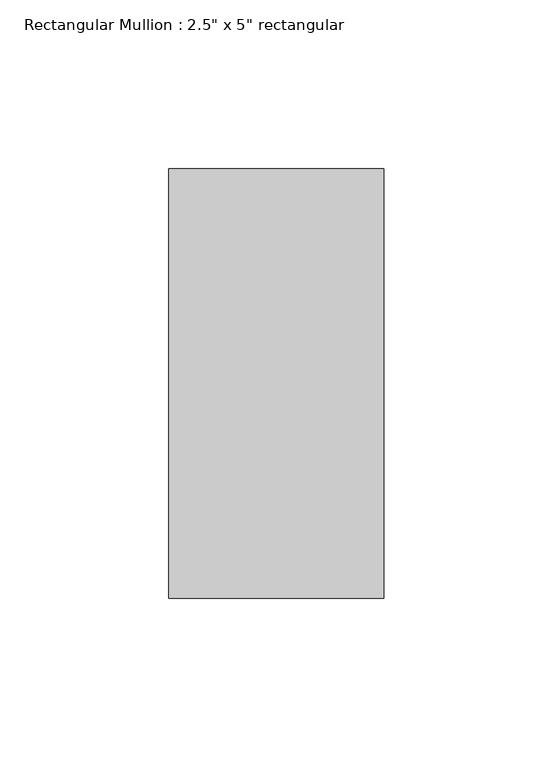
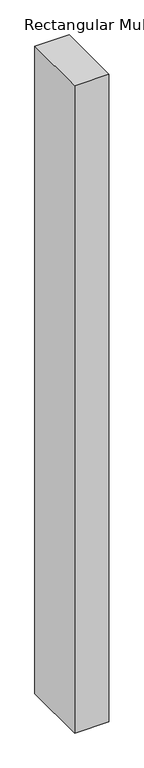
"""IFC4 building model written with IfcOpenShell, lengths in millimetres: member geometry."""

from ifc_helpers import new_model, si_unit, frame, origin, place, context, project, spatial, polyline, outline, extrude, source, transform, mapped, element, save


def member_40129ecf(model_context):
    return source(origin(), model_context, "Body", "SweptSolid", [
        extrude(outline(polyline([(31.75, 63.5), (31.75, -63.5), (-31.75, -63.5), (-31.75, 63.5), (31.75, 63.5)])), frame((0.0, 0.0, -1264.0647091), z_axis=(0.0, 0.0, 1.0), x_axis=(1.0, 0.0, 0.0)), (0.0, 0.0, 1.0), 1264.0647091),
    ])


if __name__ == "__main__":
    model = new_model("IFC4")
    model_context = context("Model", 3, world=origin())
    ifc_project = project(units=[si_unit("LENGTHUNIT", "METRE", prefix="MILLI")], contexts=[model_context])
    site = spatial("IfcSite", under=ifc_project)
    building = spatial("IfcBuilding", under=site)
    placement = place(None, origin())
    member_shape = member_40129ecf(model_context)
    element("IfcMember", 1, ObjectType="Rectangular Mullion : 2.5\" x 5\" rectangular", at=placement, inside=building, context=model_context, shape_type="MappedRepresentation", body=[
        mapped(member_shape, transform((0.0, 0.0, 0.0), x_axis=(1.0, 0.0, 0.0), y_axis=(0.0, 1.0, 0.0), z_axis=(0.0, 0.0, 1.0))),
    ])
    save(model, "model.ifc")

# Revit data of these elements
# Type "Rectangular Mullion : 2.5\" x 5\" rectangular"
#   built-in parameter 1007304 = 0.416667 (stored number, unit not read)
#   built-in parameter 1007301 = 0.104167 (stored number, unit not read)
#   built-in parameter 1007300 = 0.104167 (stored number, unit not read)
